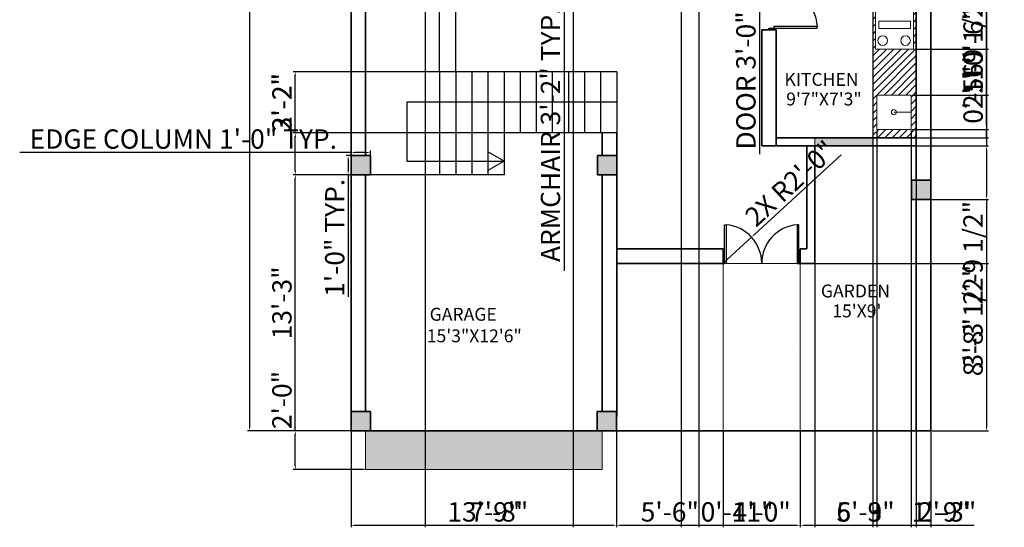
# Model space of a CAD drawing. Units: inches. Extents: x 2430 to 3058, y 1630 to 2396.
# Tile 1 of 4: x 2430 to 3042, y 1630 to 1945. Entities that reach past the tile are written whole.
import ezdxf

# ---------------------------------------------------------------- set-up
doc = ezdxf.new("R2010")
doc.units = ezdxf.units.IN
for name, color, linetype, lineweight in [('A-ANNO-DIMS', 7, 'Continuous', 18), ('A-AREA-IDEN', 131, 'Continuous', 18), ('A-COLS', 7, 'Continuous', 35), ('A-COLS-PATT', 1, 'Continuous', 13), ('A-DOOR', 40, 'Continuous', 25), ('A-FLOR-CASE', 7, 'Continuous', 25), ('A-FLOR-CASE-PATT', 131, 'Continuous', 13), ('A-FLOR-FIXT', 2, 'Continuous', 18), ('A-FLOR-STRS', 7, 'Continuous', 25), ('A-GLAZ', 131, 'Continuous', 18), ('A-GLAZ-PATT', 131, 'Continuous', 13), ('A-WALL', 7, 'Continuous', 35), ('L-PVMT', 7, 'Continuous', 18)]:
    doc.layers.add(name, color=color, linetype=linetype, lineweight=lineweight)
doc.layers.add('A-EQPM', color=33, linetype='Continuous', lineweight=18, true_color=0xb0a07d)
doc.layers.add('L-PVMT-PATT', color=241, linetype='Continuous', lineweight=13, true_color=0xf7abae)
doc.styles.get("Standard").update_dxf_attribs({"font": 'arial.ttf'})
doc.dimstyles.new('ISO-25', dxfattribs={"dimtxt": 12, "dimasz": 2.5, "dimexe": 1.25, "dimexo": 0.625, "dimtad": 1, "dimdec": 0, "dimlunit": 3, "dimtxsty": 'Standard', "dimcen": 2.5, "dimadec": 0, "dimazin": 0, "dimtfac": 1, "dimtdec": 0, "dimtmove": 0, "dimatfit": 3, "dimfxl": 1, "dimarcsym": 0})

# ---------------------------------------------------------------- blocks, each defined once
blk = doc.blocks.new('*D2')
at = {"layer": 'A-ANNO-DIMS', "color": 0, "lineweight": -2, "transparency": 16777216}
for p, q in [((2635.37, 2289.88), (2571.77, 2289.88)), ((2573.02, 2287.38), (2573.02, 1692.38)), ((2635.37, 1689.88), (2571.77, 1689.88))]:
    blk.add_line(p, q, dxfattribs=at)
at = {"layer": 'A-ANNO-DIMS', "color": 0, "transparency": 16777216}
for points in [[(2572.61, 2287.38), (2573.44, 2287.38), (2573.02, 2289.88)], [(2572.61, 1692.38), (2573.44, 1692.38), (2573.02, 1689.88)]]:
    blk.add_solid(points, dxfattribs=at)
at = {"layer": 'Defpoints', "color": 0, "transparency": 16777216}
for p in [(2636, 2289.88), (2573.02, 1689.88), (2636, 1689.88)]:
    blk.add_point(p, dxfattribs=at)
at = {"layer": 'A-ANNO-DIMS', "color": 0, "transparency": 16777216, "insert": (2566.27, 1989.88), "char_height": 12, "attachment_point": 5, "rotation": 90}
blk.add_mtext("50'", dxfattribs=at)
blk = doc.blocks.new('DOOR-30')
for p, q in [((0, 30), (0, 29)), ((0, 29), (30, 29)), ((3, 28), (3, 30)), ((30, 28), (3, 28)), ((30, 29), (30, 28)), ((0, 0), (0, 1)), ((0, 1), (3, 1)), ((3, 1), (3, 0))]:
    blk.add_line(p, q)
blk.add_arc((0.14, 30.86), 30, 275.47639, 354.52361)
blk = doc.blocks.new('COL-12x12-EDGE')
for p, q in [((12, 12), (0, 12)), ((0, 12), (0, 0)), ((0, 0), (12, 0))]:
    blk.add_line(p, q)
blk = doc.blocks.new('*D11')
at = {"layer": 'A-ANNO-DIMS', "color": 0, "lineweight": -2, "transparency": 16777216}
for p, q in [((2636, 1862.68), (2430.26, 1862.68)), ((2636, 1861.5), (2636, 1863.93)), ((2645.5, 1862.68), (2638.5, 1862.68)), ((2648, 1861.5), (2648, 1863.93))]:
    blk.add_line(p, q, dxfattribs=at)
at = {"layer": 'A-ANNO-DIMS', "color": 0, "transparency": 16777216}
for points in [[(2638.5, 1863.09), (2638.5, 1862.26), (2636, 1862.68)], [(2645.5, 1863.09), (2645.5, 1862.26), (2648, 1862.68)]]:
    blk.add_solid(points, dxfattribs=at)
at = {"layer": 'Defpoints', "color": 0, "transparency": 16777216}
for p in [(2636, 1862.68), (2636, 1860.88), (2648, 1860.88)]:
    blk.add_point(p, dxfattribs=at)
at = {"layer": 'A-ANNO-DIMS', "color": 0, "transparency": 16777216, "insert": (2531.88, 1869.51), "char_height": 12, "attachment_point": 5}
blk.add_mtext('EDGE COLUMN 1\'-0" TYP.', dxfattribs=at)
blk = doc.blocks.new('*D12')
at = {"layer": 'A-ANNO-DIMS', "color": 0, "lineweight": -2, "transparency": 16777216}
for p, q in [((2635.37, 1860.88), (2632.95, 1860.88)), ((2634.2, 1858.38), (2634.2, 1851.38)), ((2635.37, 1848.88), (2632.95, 1848.88)), ((2634.2, 1848.88), (2634.2, 1773.11))]:
    blk.add_line(p, q, dxfattribs=at)
at = {"layer": 'A-ANNO-DIMS', "color": 0, "transparency": 16777216}
for points in [[(2633.78, 1858.38), (2634.61, 1858.38), (2634.2, 1860.88)], [(2633.78, 1851.38), (2634.61, 1851.38), (2634.2, 1848.88)]]:
    blk.add_solid(points, dxfattribs=at)
at = {"layer": 'Defpoints', "color": 0, "transparency": 16777216}
for p in [(2636, 1860.88), (2634.2, 1848.88), (2636, 1848.88)]:
    blk.add_point(p, dxfattribs=at)
at = {"layer": 'A-ANNO-DIMS', "color": 0, "transparency": 16777216, "insert": (2627.44, 1809.74), "char_height": 12, "attachment_point": 5, "rotation": 90}
blk.add_mtext('1\'-0" TYP.', dxfattribs=at)
blk = doc.blocks.new('*D19')
at = {"layer": 'A-ANNO-DIMS', "color": 0, "lineweight": -2, "transparency": 16777216}
for p, q in [((2894.37, 2028.88), (2888.35, 2028.88)), ((2889.6, 2026.38), (2889.6, 1995.38)), ((2894.37, 1992.88), (2888.35, 1992.88)), ((2889.6, 1992.88), (2889.6, 1861.63))]:
    blk.add_line(p, q, dxfattribs=at)
at = {"layer": 'A-ANNO-DIMS', "color": 0, "transparency": 16777216}
for points in [[(2889.18, 2026.38), (2890.01, 2026.38), (2889.6, 2028.88)], [(2889.18, 1995.38), (2890.01, 1995.38), (2889.6, 1992.88)]]:
    blk.add_solid(points, dxfattribs=at)
at = {"layer": 'Defpoints', "color": 0, "transparency": 16777216}
for p in [(2895, 2028.88), (2889.6, 1992.88), (2895, 1992.88)]:
    blk.add_point(p, dxfattribs=at)
at = {"layer": 'A-ANNO-DIMS', "color": 0, "transparency": 16777216, "insert": (2882.76, 1926), "char_height": 12, "attachment_point": 5, "rotation": 90}
blk.add_mtext('DOOR 3\'-0" TYP.', dxfattribs=at)
blk = doc.blocks.new('*D25')
at = {"layer": 'A-ANNO-DIMS', "color": 0, "lineweight": -2, "transparency": 16777216}
for p, q in [((2773.33, 1998.82), (2767, 1998.82)), ((2768.25, 1996.32), (2768.25, 1963.32)), ((2773.33, 1960.82), (2767, 1960.82)), ((2768.25, 1960.82), (2768.25, 1789.16))]:
    blk.add_line(p, q, dxfattribs=at)
at = {"layer": 'A-ANNO-DIMS', "color": 0, "transparency": 16777216}
for points in [[(2767.83, 1996.32), (2768.67, 1996.32), (2768.25, 1998.82)], [(2767.83, 1963.32), (2768.67, 1963.32), (2768.25, 1960.82)]]:
    blk.add_solid(points, dxfattribs=at)
at = {"layer": 'Defpoints', "color": 0, "transparency": 16777216}
for p in [(2773.95, 1998.82), (2768.25, 1960.82), (2773.95, 1960.82)]:
    blk.add_point(p, dxfattribs=at)
at = {"layer": 'A-ANNO-DIMS', "color": 0, "transparency": 16777216, "insert": (2761.42, 1873.74), "char_height": 12, "attachment_point": 5, "rotation": 90}
blk.add_mtext('ARMCHAIR 3\'-2" TYP.', dxfattribs=at)
blk = doc.blocks.new('*D32')
at = {"layer": 'A-ANNO-DIMS', "color": 0, "lineweight": -2, "transparency": 16777216}
for p, q in [((2996.62, 1992.88), (3031.85, 1992.88)), ((3030.6, 1990.38), (3030.6, 1869.38)), ((2987.62, 1866.88), (3031.85, 1866.88))]:
    blk.add_line(p, q, dxfattribs=at)
at = {"layer": 'A-ANNO-DIMS', "color": 0, "transparency": 16777216}
for points in [[(3030.18, 1990.38), (3031.01, 1990.38), (3030.6, 1992.88)], [(3030.18, 1869.38), (3031.01, 1869.38), (3030.6, 1866.88)]]:
    blk.add_solid(points, dxfattribs=at)
at = {"layer": 'Defpoints', "color": 0, "transparency": 16777216}
for p in [(2996, 1992.88), (2987, 1866.88), (3030.6, 1866.88)]:
    blk.add_point(p, dxfattribs=at)
at = {"layer": 'A-ANNO-DIMS', "color": 0, "transparency": 16777216, "insert": (3023.84, 1929.88), "char_height": 12, "attachment_point": 5, "rotation": 90}
blk.add_mtext('10\'-6"', dxfattribs=at)
blk = doc.blocks.new('*D33')
at = {"layer": 'A-ANNO-DIMS', "color": 0, "lineweight": -2, "transparency": 16777216}
for p, q in [((2987.62, 1866.88), (3031.85, 1866.88)), ((3030.6, 1864.38), (3030.6, 1836.1)), ((2996.62, 1833.6), (3031.85, 1833.6)), ((3030.6, 1833.6), (3030.6, 1769.78))]:
    blk.add_line(p, q, dxfattribs=at)
at = {"layer": 'A-ANNO-DIMS', "color": 0, "transparency": 16777216}
for points in [[(3030.18, 1864.38), (3031.01, 1864.38), (3030.6, 1866.88)], [(3030.18, 1836.1), (3031.01, 1836.1), (3030.6, 1833.6)]]:
    blk.add_solid(points, dxfattribs=at)
at = {"layer": 'Defpoints', "color": 0, "transparency": 16777216}
for p in [(2987, 1866.88), (2996, 1833.6), (3030.6, 1833.6)]:
    blk.add_point(p, dxfattribs=at)
at = {"layer": 'A-ANNO-DIMS', "color": 0, "transparency": 16777216, "insert": (3023.77, 1800.44), "char_height": 12, "attachment_point": 5, "rotation": 90}
blk.add_mtext('2\'-9 1/2"', dxfattribs=at)
blk = doc.blocks.new('*D34')
at = {"layer": 'A-ANNO-DIMS', "color": 0, "lineweight": -2, "transparency": 16777216}
for p, q in [((2996.62, 1833.6), (3031.85, 1833.6)), ((3030.6, 1831.1), (3030.6, 1796.38)), ((2924.62, 1793.88), (3031.85, 1793.88)), ((3030.6, 1793.88), (3030.6, 1730.28))]:
    blk.add_line(p, q, dxfattribs=at)
at = {"layer": 'A-ANNO-DIMS', "color": 0, "transparency": 16777216}
for points in [[(3030.18, 1831.1), (3031.01, 1831.1), (3030.6, 1833.6)], [(3030.18, 1796.38), (3031.01, 1796.38), (3030.6, 1793.88)]]:
    blk.add_solid(points, dxfattribs=at)
at = {"layer": 'Defpoints', "color": 0, "transparency": 16777216}
for p in [(2996, 1833.6), (2924, 1793.88), (3030.6, 1793.88)]:
    blk.add_point(p, dxfattribs=at)
at = {"layer": 'A-ANNO-DIMS', "color": 0, "transparency": 16777216, "insert": (3023.76, 1760.83), "char_height": 12, "attachment_point": 5, "rotation": 90}
blk.add_mtext('3\'-3 1/2"', dxfattribs=at)
blk = doc.blocks.new('*D35')
at = {"layer": 'A-ANNO-DIMS', "color": 0, "lineweight": -2, "transparency": 16777216}
for p, q in [((2924.62, 1793.88), (3031.85, 1793.88)), ((3030.6, 1791.38), (3030.6, 1692.38)), ((2996.62, 1689.88), (3031.85, 1689.88))]:
    blk.add_line(p, q, dxfattribs=at)
at = {"layer": 'A-ANNO-DIMS', "color": 0, "transparency": 16777216}
for points in [[(3030.18, 1791.38), (3031.01, 1791.38), (3030.6, 1793.88)], [(3030.18, 1692.38), (3031.01, 1692.38), (3030.6, 1689.88)]]:
    blk.add_solid(points, dxfattribs=at)
at = {"layer": 'Defpoints', "color": 0, "transparency": 16777216}
for p in [(2924, 1793.88), (2996, 1689.88), (3030.6, 1689.88)]:
    blk.add_point(p, dxfattribs=at)
at = {"layer": 'A-ANNO-DIMS', "color": 0, "transparency": 16777216, "insert": (3023.84, 1741.88), "char_height": 12, "attachment_point": 5, "rotation": 90}
blk.add_mtext('8\'-8"', dxfattribs=at)
blk = doc.blocks.new('*D36')
at = {"layer": 'A-ANNO-DIMS', "color": 0, "lineweight": -2, "transparency": 16777216}
for p, q in [((2635.37, 1848.88), (2600.15, 1848.88)), ((2601.4, 1692.38), (2601.4, 1846.38)), ((2635.37, 1689.88), (2600.15, 1689.88))]:
    blk.add_line(p, q, dxfattribs=at)
at = {"layer": 'A-ANNO-DIMS', "color": 0, "transparency": 16777216}
for points in [[(2600.98, 1846.38), (2601.81, 1846.38), (2601.4, 1848.88)], [(2600.98, 1692.38), (2601.81, 1692.38), (2601.4, 1689.88)]]:
    blk.add_solid(points, dxfattribs=at)
at = {"layer": 'Defpoints', "color": 0, "transparency": 16777216}
for p in [(2601.4, 1848.88), (2636, 1848.88), (2636, 1689.88)]:
    blk.add_point(p, dxfattribs=at)
at = {"layer": 'A-ANNO-DIMS', "color": 0, "transparency": 16777216, "insert": (2594.64, 1769.38), "char_height": 12, "attachment_point": 5, "rotation": 90}
blk.add_mtext('13\'-3"', dxfattribs=at)
blk = doc.blocks.new('*D37')
at = {"layer": 'A-ANNO-DIMS', "color": 0, "lineweight": -2, "transparency": 16777216}
for p, q in [((2601.4, 1689.88), (2601.4, 1725.73)), ((2644.37, 1689.88), (2600.15, 1689.88)), ((2601.4, 1668.38), (2601.4, 1687.38)), ((2644.37, 1665.88), (2600.15, 1665.88))]:
    blk.add_line(p, q, dxfattribs=at)
at = {"layer": 'A-ANNO-DIMS', "color": 0, "transparency": 16777216}
for points in [[(2600.98, 1687.38), (2601.81, 1687.38), (2601.4, 1689.88)], [(2600.98, 1668.38), (2601.81, 1668.38), (2601.4, 1665.88)]]:
    blk.add_solid(points, dxfattribs=at)
at = {"layer": 'Defpoints', "color": 0, "transparency": 16777216}
for p in [(2601.4, 1689.88), (2645, 1689.88), (2645, 1665.88)]:
    blk.add_point(p, dxfattribs=at)
at = {"layer": 'A-ANNO-DIMS', "color": 0, "transparency": 16777216, "insert": (2594.64, 1709.05), "char_height": 12, "attachment_point": 5, "rotation": 90}
blk.add_mtext('2\'-0"', dxfattribs=at)
blk = doc.blocks.new('*D38')
at = {"layer": 'A-ANNO-DIMS', "color": 0, "lineweight": -2, "transparency": 16777216}
for p, q in [((2636, 1689.25), (2636, 1630.03)), ((2800.92, 1689.25), (2800.92, 1630.03)), ((2638.5, 1631.28), (2798.42, 1631.28))]:
    blk.add_line(p, q, dxfattribs=at)
at = {"layer": 'A-ANNO-DIMS', "color": 0, "transparency": 16777216}
for points in [[(2638.5, 1631.69), (2638.5, 1630.86), (2636, 1631.28)], [(2798.42, 1631.69), (2798.42, 1630.86), (2800.92, 1631.28)]]:
    blk.add_solid(points, dxfattribs=at)
at = {"layer": 'Defpoints', "color": 0, "transparency": 16777216}
for p in [(2636, 1689.88), (2800.92, 1689.88), (2800.92, 1631.28)]:
    blk.add_point(p, dxfattribs=at)
at = {"layer": 'A-ANNO-DIMS', "color": 0, "transparency": 16777216, "insert": (2718.46, 1638.03), "char_height": 12, "attachment_point": 5}
blk.add_mtext('13\'-9"', dxfattribs=at)
blk = doc.blocks.new('*D39')
at = {"layer": 'A-ANNO-DIMS', "color": 0, "lineweight": -2, "transparency": 16777216}
for p, q in [((2800.92, 1689.25), (2800.92, 1630.03)), ((2867, 1689.25), (2867, 1630.03)), ((2803.42, 1631.28), (2864.5, 1631.28))]:
    blk.add_line(p, q, dxfattribs=at)
at = {"layer": 'A-ANNO-DIMS', "color": 0, "transparency": 16777216}
for points in [[(2803.42, 1631.69), (2803.42, 1630.86), (2800.92, 1631.28)], [(2864.5, 1631.69), (2864.5, 1630.86), (2867, 1631.28)]]:
    blk.add_solid(points, dxfattribs=at)
at = {"layer": 'Defpoints', "color": 0, "transparency": 16777216}
for p in [(2800.92, 1689.88), (2867, 1689.88), (2867, 1631.28)]:
    blk.add_point(p, dxfattribs=at)
at = {"layer": 'A-ANNO-DIMS', "color": 0, "transparency": 16777216, "insert": (2833.96, 1638.03), "char_height": 12, "attachment_point": 5}
blk.add_mtext('5\'-6"', dxfattribs=at)
blk = doc.blocks.new('*D40')
at = {"layer": 'A-ANNO-DIMS', "color": 0, "lineweight": -2, "transparency": 16777216}
for p, q in [((2867, 1689.25), (2867, 1630.03)), ((2915, 1689.25), (2915, 1630.03)), ((2869.5, 1631.28), (2912.5, 1631.28))]:
    blk.add_line(p, q, dxfattribs=at)
at = {"layer": 'A-ANNO-DIMS', "color": 0, "transparency": 16777216}
for points in [[(2869.5, 1631.69), (2869.5, 1630.86), (2867, 1631.28)], [(2912.5, 1631.69), (2912.5, 1630.86), (2915, 1631.28)]]:
    blk.add_solid(points, dxfattribs=at)
at = {"layer": 'Defpoints', "color": 0, "transparency": 16777216}
for p in [(2867, 1689.88), (2915, 1689.88), (2915, 1631.28)]:
    blk.add_point(p, dxfattribs=at)
at = {"layer": 'A-ANNO-DIMS', "color": 0, "transparency": 16777216, "insert": (2891, 1638.03), "char_height": 12, "attachment_point": 5}
blk.add_mtext('4\'-0"', dxfattribs=at)
blk = doc.blocks.new('*D41')
at = {"layer": 'A-ANNO-DIMS', "color": 0, "lineweight": -2, "transparency": 16777216}
for p, q in [((2915, 1689.25), (2915, 1630.03)), ((2996, 1689.25), (2996, 1630.03)), ((2917.5, 1631.28), (2993.5, 1631.28))]:
    blk.add_line(p, q, dxfattribs=at)
at = {"layer": 'A-ANNO-DIMS', "color": 0, "transparency": 16777216}
for points in [[(2917.5, 1631.69), (2917.5, 1630.86), (2915, 1631.28)], [(2993.5, 1631.69), (2993.5, 1630.86), (2996, 1631.28)]]:
    blk.add_solid(points, dxfattribs=at)
at = {"layer": 'Defpoints', "color": 0, "transparency": 16777216}
for p in [(2915, 1689.88), (2996, 1689.88), (2996, 1631.28)]:
    blk.add_point(p, dxfattribs=at)
at = {"layer": 'A-ANNO-DIMS', "color": 0, "transparency": 16777216, "insert": (2955.5, 1638.03), "char_height": 12, "attachment_point": 5}
blk.add_mtext('6\'-9"', dxfattribs=at)
blk = doc.blocks.new('*D42')
at = {"layer": 'A-ANNO-DIMS', "color": 0, "lineweight": -2, "transparency": 16777216}
for p, q in [((2601.4, 1874.88), (2601.4, 1910.73)), ((2644.37, 1874.88), (2600.15, 1874.88)), ((2601.4, 1851.38), (2601.4, 1872.38)), ((2644.37, 1848.88), (2600.15, 1848.88))]:
    blk.add_line(p, q, dxfattribs=at)
at = {"layer": 'A-ANNO-DIMS', "color": 0, "transparency": 16777216}
for points in [[(2600.98, 1872.38), (2601.81, 1872.38), (2601.4, 1874.88)], [(2600.98, 1851.38), (2601.81, 1851.38), (2601.4, 1848.88)]]:
    blk.add_solid(points, dxfattribs=at)
at = {"layer": 'Defpoints', "color": 0, "transparency": 16777216}
for p in [(2601.4, 1874.88), (2645, 1874.88), (2645, 1848.88)]:
    blk.add_point(p, dxfattribs=at)
at = {"layer": 'A-ANNO-DIMS', "color": 0, "transparency": 16777216, "insert": (2594.75, 1894.05), "char_height": 12, "attachment_point": 5, "rotation": 90}
blk.add_mtext('2\'-2"', dxfattribs=at)
blk = doc.blocks.new('*D43')
at = {"layer": 'A-ANNO-DIMS', "color": 0, "lineweight": -2, "transparency": 16777216}
for p, q in [((2644.37, 1912.88), (2600.15, 1912.88)), ((2601.4, 1877.38), (2601.4, 1910.38)), ((2644.37, 1874.88), (2600.15, 1874.88))]:
    blk.add_line(p, q, dxfattribs=at)
at = {"layer": 'A-ANNO-DIMS', "color": 0, "transparency": 16777216}
for points in [[(2600.98, 1910.38), (2601.81, 1910.38), (2601.4, 1912.88)], [(2600.98, 1877.38), (2601.81, 1877.38), (2601.4, 1874.88)]]:
    blk.add_solid(points, dxfattribs=at)
at = {"layer": 'Defpoints', "color": 0, "transparency": 16777216}
for p in [(2601.4, 1912.88), (2645, 1912.88), (2645, 1874.88)]:
    blk.add_point(p, dxfattribs=at)
at = {"layer": 'A-ANNO-DIMS', "color": 0, "transparency": 16777216, "insert": (2594.64, 1893.88), "char_height": 12, "attachment_point": 5, "rotation": 90}
blk.add_mtext('3\'-2"', dxfattribs=at)
blk = doc.blocks.new('*D44')
at = {"layer": 'A-ANNO-DIMS', "color": 0, "lineweight": -2, "transparency": 16777216}
for p, q in [((2691, 1913.5), (2691, 2325.73)), ((2693.5, 2324.48), (2698.5, 2324.48)), ((2701, 1913.5), (2701, 2325.73)), ((2701, 2324.48), (2745.97, 2324.48))]:
    blk.add_line(p, q, dxfattribs=at)
at = {"layer": 'A-ANNO-DIMS', "color": 0, "transparency": 16777216}
for points in [[(2693.5, 2324.89), (2693.5, 2324.06), (2691, 2324.48)], [(2698.5, 2324.89), (2698.5, 2324.06), (2701, 2324.48)]]:
    blk.add_solid(points, dxfattribs=at)
at = {"layer": 'Defpoints', "color": 0, "transparency": 16777216}
for p in [(2701, 2324.48), (2691, 1912.88), (2701, 1912.88)]:
    blk.add_point(p, dxfattribs=at)
at = {"layer": 'A-ANNO-DIMS', "color": 0, "transparency": 16777216, "insert": (2724.73, 2331.23), "char_height": 12, "attachment_point": 5}
blk.add_mtext('0\'-10"', dxfattribs=at)
blk = doc.blocks.new('*D45')
at = {"layer": 'A-ANNO-DIMS', "color": 0, "lineweight": -2, "transparency": 16777216}
for p, q in [((2924, 1866.25), (2924, 1630.03)), ((2987, 1866.25), (2987, 1630.03)), ((2926.5, 1631.28), (2984.5, 1631.28))]:
    blk.add_line(p, q, dxfattribs=at)
at = {"layer": 'A-ANNO-DIMS', "color": 0, "transparency": 16777216}
for points in [[(2926.5, 1631.69), (2926.5, 1630.86), (2924, 1631.28)], [(2984.5, 1631.69), (2984.5, 1630.86), (2987, 1631.28)]]:
    blk.add_solid(points, dxfattribs=at)
at = {"layer": 'Defpoints', "color": 0, "transparency": 16777216}
for p in [(2924, 1866.88), (2987, 1866.88), (2987, 1631.28)]:
    blk.add_point(p, dxfattribs=at)
at = {"layer": 'A-ANNO-DIMS', "color": 0, "transparency": 16777216, "insert": (2955.5, 1638.03), "char_height": 12, "attachment_point": 5}
blk.add_mtext('5\'-3"', dxfattribs=at)
blk = doc.blocks.new('*D49')
at = {"layer": 'A-ANNO-DIMS', "color": 0, "lineweight": -2, "transparency": 16777216}
for p, q in [((2840.99, 2130.25), (2840.99, 1630.03)), ((2852, 2130.25), (2852, 1630.03)), ((2843.49, 1631.28), (2849.5, 1631.28)), ((2852, 1631.28), (2896.97, 1631.28))]:
    blk.add_line(p, q, dxfattribs=at)
at = {"layer": 'A-ANNO-DIMS', "color": 0, "transparency": 16777216}
for points in [[(2843.49, 1631.69), (2843.49, 1630.86), (2840.99, 1631.28)], [(2849.5, 1631.69), (2849.5, 1630.86), (2852, 1631.28)]]:
    blk.add_solid(points, dxfattribs=at)
at = {"layer": 'Defpoints', "color": 0, "transparency": 16777216}
for p in [(2840.99, 2130.88), (2852, 2130.88), (2852, 1631.28)]:
    blk.add_point(p, dxfattribs=at)
at = {"layer": 'A-ANNO-DIMS', "color": 0, "transparency": 16777216, "insert": (2875.73, 1638.03), "char_height": 12, "attachment_point": 5}
blk.add_mtext('0\'-11"', dxfattribs=at)
blk = doc.blocks.new('*D50')
at = {"layer": 'A-ANNO-DIMS', "color": 0, "lineweight": -2, "transparency": 16777216}
for p, q in [((2960, 1871.25), (2960, 1630.03)), ((2987, 1871.25), (2987, 1630.03)), ((2962.5, 1631.28), (2984.5, 1631.28)), ((2987, 1631.28), (3022.85, 1631.28))]:
    blk.add_line(p, q, dxfattribs=at)
at = {"layer": 'A-ANNO-DIMS', "color": 0, "transparency": 16777216}
for points in [[(2962.5, 1631.69), (2962.5, 1630.86), (2960, 1631.28)], [(2984.5, 1631.69), (2984.5, 1630.86), (2987, 1631.28)]]:
    blk.add_solid(points, dxfattribs=at)
at = {"layer": 'Defpoints', "color": 0, "transparency": 16777216}
for p in [(2960, 1871.88), (2987, 1871.88), (2987, 1631.28)]:
    blk.add_point(p, dxfattribs=at)
at = {"layer": 'A-ANNO-DIMS', "color": 0, "transparency": 16777216, "insert": (3006.17, 1638.03), "char_height": 12, "attachment_point": 5}
blk.add_mtext('2\'-3"', dxfattribs=at)
blk = doc.blocks.new('*D53')
at = {"layer": 'A-ANNO-DIMS', "color": 0, "lineweight": -2, "transparency": 16777216}
for p, q in [((2985.92, 1956.85), (3031.85, 1956.85)), ((3030.6, 1954.35), (3030.6, 1929.42)), ((2985.92, 1926.92), (3031.85, 1926.92)), ((3030.6, 1926.92), (3030.6, 1891.07))]:
    blk.add_line(p, q, dxfattribs=at)
at = {"layer": 'A-ANNO-DIMS', "color": 0, "transparency": 16777216}
for points in [[(3030.18, 1954.35), (3031.01, 1954.35), (3030.6, 1956.85)], [(3030.18, 1929.42), (3031.01, 1929.42), (3030.6, 1926.92)]]:
    blk.add_solid(points, dxfattribs=at)
at = {"layer": 'Defpoints', "color": 0, "transparency": 16777216}
for p in [(2985.3, 1956.85), (2985.3, 1926.92), (3030.6, 1926.92)]:
    blk.add_point(p, dxfattribs=at)
at = {"layer": 'A-ANNO-DIMS', "color": 0, "transparency": 16777216, "insert": (3023.84, 1907.75), "char_height": 12, "attachment_point": 5, "rotation": 90}
blk.add_mtext('2\'-6"', dxfattribs=at)
blk = doc.blocks.new('*D54')
at = {"layer": 'A-ANNO-DIMS', "color": 0, "lineweight": -2, "transparency": 16777216}
for p, q in [((2962.55, 1876.44), (2962.55, 1630.03)), ((2983.75, 1876.44), (2983.75, 1630.03)), ((2965.05, 1631.28), (2981.25, 1631.28)), ((2983.75, 1631.28), (3018.27, 1631.28))]:
    blk.add_line(p, q, dxfattribs=at)
at = {"layer": 'A-ANNO-DIMS', "color": 0, "transparency": 16777216}
for points in [[(2965.05, 1631.69), (2965.05, 1630.86), (2962.55, 1631.28)], [(2981.25, 1631.69), (2981.25, 1630.86), (2983.75, 1631.28)]]:
    blk.add_solid(points, dxfattribs=at)
at = {"layer": 'Defpoints', "color": 0, "transparency": 16777216}
for p in [(2962.55, 1877.06), (2983.75, 1877.06), (2983.75, 1631.28)]:
    blk.add_point(p, dxfattribs=at)
at = {"layer": 'A-ANNO-DIMS', "color": 0, "transparency": 16777216, "insert": (3002.26, 1638.03), "char_height": 12, "attachment_point": 5}
blk.add_mtext('1\'-9"', dxfattribs=at)
blk = doc.blocks.new('*D55')
at = {"layer": 'A-ANNO-DIMS', "color": 0, "lineweight": -2, "transparency": 16777216}
for p, q in [((3030.6, 1898.4), (3030.6, 1960.88)), ((2984.38, 1898.4), (3031.85, 1898.4)), ((3030.6, 1879.56), (3030.6, 1895.9)), ((2984.38, 1877.06), (3031.85, 1877.06))]:
    blk.add_line(p, q, dxfattribs=at)
at = {"layer": 'A-ANNO-DIMS', "color": 0, "transparency": 16777216}
for points in [[(3030.18, 1895.9), (3031.01, 1895.9), (3030.6, 1898.4)], [(3030.18, 1879.56), (3031.01, 1879.56), (3030.6, 1877.06)]]:
    blk.add_solid(points, dxfattribs=at)
at = {"layer": 'Defpoints', "color": 0, "transparency": 16777216}
for p in [(2983.75, 1898.4), (3030.6, 1898.4), (2983.75, 1877.06)]:
    blk.add_point(p, dxfattribs=at)
at = {"layer": 'A-ANNO-DIMS', "color": 0, "transparency": 16777216, "insert": (3023.77, 1930.89), "char_height": 12, "attachment_point": 5, "rotation": 90}
blk.add_mtext('1\'-9 1/2"', dxfattribs=at)
blk = doc.blocks.new('*D57')
at = {"layer": 'A-ANNO-DIMS', "color": 0, "lineweight": -2, "transparency": 16777216}
for p, q in [((3030.6, 1879.56), (3030.6, 1915.21)), ((2984.38, 1877.06), (3031.85, 1877.06)), ((3030.6, 1871.88), (3030.6, 1877.06)), ((2987.62, 1871.88), (3031.85, 1871.88)), ((3030.6, 1869.38), (3030.6, 1866.88))]:
    blk.add_line(p, q, dxfattribs=at)
at = {"layer": 'A-ANNO-DIMS', "color": 0, "transparency": 16777216}
for points in [[(3030.18, 1879.56), (3031.01, 1879.56), (3030.6, 1877.06)], [(3030.18, 1869.38), (3031.01, 1869.38), (3030.6, 1871.88)]]:
    blk.add_solid(points, dxfattribs=at)
at = {"layer": 'Defpoints', "color": 0, "transparency": 16777216}
for p in [(2983.75, 1877.06), (3030.6, 1877.06), (2987, 1871.88)]:
    blk.add_point(p, dxfattribs=at)
at = {"layer": 'A-ANNO-DIMS', "color": 0, "transparency": 16777216, "insert": (3023.84, 1898.64), "char_height": 12, "attachment_point": 5, "rotation": 90}
blk.add_mtext('0\'-5"', dxfattribs=at)
blk = doc.blocks.new('*D65')
at = {"layer": 'A-ANNO-DIMS', "color": 0, "lineweight": -2, "transparency": 16777216}
for p, q in [((2682, 1962.2), (2682, 1630.03)), ((2773.95, 1962.2), (2773.95, 1630.03)), ((2684.5, 1631.28), (2771.45, 1631.28))]:
    blk.add_line(p, q, dxfattribs=at)
at = {"layer": 'A-ANNO-DIMS', "color": 0, "transparency": 16777216}
for points in [[(2684.5, 1631.69), (2684.5, 1630.86), (2682, 1631.28)], [(2771.45, 1631.69), (2771.45, 1630.86), (2773.95, 1631.28)]]:
    blk.add_solid(points, dxfattribs=at)
at = {"layer": 'Defpoints', "color": 0, "transparency": 16777216}
for p in [(2682, 1962.82), (2773.95, 1962.82), (2773.95, 1631.28)]:
    blk.add_point(p, dxfattribs=at)
at = {"layer": 'A-ANNO-DIMS', "color": 0, "transparency": 16777216, "insert": (2727.97, 1638.03), "char_height": 12, "attachment_point": 5}
blk.add_mtext('7\'-8"', dxfattribs=at)
blk = doc.blocks.new('*D66')
at = {"layer": 'A-ANNO-DIMS', "color": 0, "lineweight": -2, "transparency": 16777216}
for p, q in [((2940.43, 1861.28), (2886.53, 1811.87)), ((2867, 1793.96), (2884.69, 1810.18))]:
    blk.add_line(p, q, dxfattribs=at)
at = {"layer": 'A-ANNO-DIMS', "color": 0, "transparency": 16777216}
blk.add_solid([(2886.25, 1812.18), (2886.81, 1811.56), (2884.69, 1810.18)], dxfattribs=at)
at = {"layer": 'Defpoints', "color": 0, "transparency": 16777216}
for p in [(2884.69, 1810.18), (2867, 1793.96)]:
    blk.add_point(p, dxfattribs=at)
at = {"layer": 'A-ANNO-DIMS', "color": 0, "transparency": 16777216, "insert": (2909.84, 1842.4), "char_height": 12, "attachment_point": 5, "rotation": 42.5117}
blk.add_mtext('2X R2\'-0"', dxfattribs=at)

msp = doc.modelspace()

# ---------------------------------------------------------------- hatches: boundary and pattern name
at = {"layer": 'A-COLS-PATT'}
h = msp.add_hatch(color=256, dxfattribs=at)
h.dxf.hatch_style = 1
h.paths.add_polyline_path([(2648, 1860.88), (2636, 1860.88), (2636, 1848.88), (2648, 1848.88)])
h = msp.add_hatch(color=256, dxfattribs=at)
h.dxf.hatch_style = 1
h.paths.add_polyline_path([(2801, 1860.88), (2789, 1860.88), (2789, 1848.88), (2801, 1848.88)])
h = msp.add_hatch(color=256, dxfattribs=at)
h.dxf.hatch_style = 1
h.paths.add_polyline_path([(2996, 1845.6), (2984, 1845.6), (2984, 1833.6), (2996, 1833.6)])
h = msp.add_hatch(color=256, dxfattribs=at)
h.dxf.hatch_style = 1
h.paths.add_polyline_path([(2648, 1701.88), (2636, 1701.88), (2636, 1689.88), (2648, 1689.88)])
h = msp.add_hatch(color=256, dxfattribs=at)
h.dxf.hatch_style = 1
h.paths.add_polyline_path([(2800.92, 1701.88), (2788.92, 1701.88), (2788.92, 1689.88), (2800.92, 1689.88)])
at = {"layer": 'A-FLOR-CASE-PATT'}
h = msp.add_hatch(dxfattribs=at)
h.set_pattern_fill('ANSI31', color=256)
h.paths.add_polyline_path([(2987, 1980.88), (2984, 1980.88), (2984, 1987.88), (2900, 1987.88), (2900, 1968.88), (2960, 1968.88), (2960, 1871.88), (2987, 1871.88)])
h.paths.add_polyline_path([(2961.68, 1956.85), (2985.3, 1956.85), (2985.3, 1926.92), (2961.68, 1926.92)], flags=16)
h.paths.add_polyline_path([(2969.08, 1951.68, -1), (2963.08, 1951.68, -1)], flags=0)
h.paths.add_polyline_path([(2963.83, 1944.18), (2983.44, 1944.18), (2983.44, 1939.79), (2963.83, 1939.79)], flags=0)
h.paths.add_polyline_path([(2983.32, 1951.68, -1), (2977.32, 1951.68, -1)], flags=0)
h.paths.add_polyline_path([(2969.08, 1932.19, -1), (2963.08, 1932.19, -1)], flags=0)
h.paths.add_polyline_path([(2983.32, 1932.19, -1), (2977.32, 1932.19, -1)], flags=0)
h.paths.add_polyline_path([(2962.55, 1898.4), (2983.75, 1898.4), (2983.75, 1877.06), (2962.55, 1877.06)], flags=16)
h.paths.add_polyline_path([(2974.72, 1887.73, -1), (2971.58, 1887.73, -1)], flags=0)
at = {"layer": 'A-GLAZ-PATT'}
h = msp.add_hatch(color=256, dxfattribs=at)
h.dxf.hatch_style = 1
h.paths.add_polyline_path([(2960, 1871.88), (2924, 1871.88), (2924, 1866.88), (2960, 1866.88)])
at = {"layer": 'L-PVMT-PATT'}
h = msp.add_hatch(dxfattribs=at)
h.set_pattern_fill('AR-CONC', color=256)
h.paths.add_polyline_path([(2915, 1793.88), (2914, 1793.88), (2913, 1793.88), (2867, 1793.88), (2867, 1698.88), (2915, 1698.88)])
h = msp.add_hatch(color=256, dxfattribs=at)
h.dxf.hatch_style = 1
h.paths.add_polyline_path([(2792, 1689.88), (2645, 1689.88), (2645, 1665.88), (2792, 1665.88)])

# ---------------------------------------------------------------- linework, layer by layer
at = {"layer": 'A-COLS'}
for p, q in [((2789, 1848.88), (2789, 1860.88)), ((2789, 1860.88), (2801, 1860.88)), ((2801, 1848.88), (2789, 1848.88)), ((2801, 1848.88), (2789, 1848.88))]:
    msp.add_line(p, q, dxfattribs=at)
at = {"layer": 'A-DOOR'}
for p, q in [((2868, 1793.88), (2868, 1817.88)), ((2868, 1817.88), (2869, 1817.88)), ((2869, 1817.88), (2869, 1793.88)), ((2914, 1817.88), (2913, 1817.88)), ((2913, 1817.88), (2913, 1793.88)), ((2914, 1793.88), (2914, 1817.88)), ((2867, 1793.88), (2868, 1793.88)), ((2869, 1793.88), (2867, 1793.88)), ((2913, 1793.88), (2914.5, 1793.88)), ((2915, 1793.88), (2914, 1793.88))]:
    msp.add_line(p, q, dxfattribs=at)
for centre, start, end in [((2867, 1793.96), 359.80074, 85.22016), ((2915, 1793.96), 94.77984, 180.19926)]:
    msp.add_arc(centre, 24, start, end, dxfattribs=at)
at = {"layer": 'A-EQPM'}
for points in [[(2961.68, 1956.85), (2985.3, 1956.85), (2985.3, 1926.92), (2961.68, 1926.92)], [(2963.83, 1944.18), (2983.44, 1944.18), (2983.44, 1939.79), (2963.83, 1939.79)]]:
    msp.add_lwpolyline(points, close=True, dxfattribs=at)
for centre in [(2966.08, 1932.19), (2980.32, 1932.19)]:
    msp.add_circle(centre, 3, dxfattribs=at)
at = {"layer": 'A-FLOR-CASE'}
msp.add_line((2960, 1968.88), (2960, 1871.88), dxfattribs=at)
at = {"layer": 'A-FLOR-FIXT'}
msp.add_line((2973.15, 1887.73), (2983.75, 1887.73), dxfattribs=at)
msp.add_lwpolyline([(2962.55, 1898.4), (2983.75, 1898.4), (2983.75, 1877.06), (2962.55, 1877.06)], close=True, dxfattribs=at)
msp.add_circle((2973.15, 1887.73), 1.57, dxfattribs=at)
at = {"layer": 'A-FLOR-STRS'}
for p, q in [((2801, 1912.88), (2645, 1912.88)), ((2691, 1912.88), (2691, 1848.88)), ((2701, 1912.88), (2701, 1848.88)), ((2711, 1912.88), (2711, 1848.88)), ((2721, 1912.88), (2721, 1848.88)), ((2731, 1912.88), (2731, 1848.88)), ((2741, 1912.88), (2741, 1874.88)), ((2751, 1912.88), (2751, 1874.88)), ((2761, 1912.88), (2761, 1874.88)), ((2771, 1912.88), (2771, 1874.88)), ((2781, 1912.88), (2781, 1874.88)), ((2791, 1912.88), (2791, 1874.88)), ((2801, 1912.88), (2801, 1874.88)), ((2801, 1893.88), (2670.61, 1893.88)), ((2670.61, 1893.88), (2670.61, 1857.36)), ((2801, 1874.88), (2645, 1874.88)), ((2731, 1857.36), (2721, 1863.14)), ((2670.61, 1857.36), (2731, 1857.36)), ((2731, 1857.36), (2721, 1851.59)), ((2731, 1848.88), (2645, 1848.88))]:
    msp.add_line(p, q, dxfattribs=at)
at = {"layer": 'A-GLAZ'}
for p, q in [((2924, 1871.88), (2924, 1866.88)), ((2960, 1871.88), (2960, 1866.88))]:
    msp.add_line(p, q, dxfattribs=at)
at = {"layer": 'A-WALL'}
for p, q in [((2645, 1860.88), (2645, 1989.88)), ((2987, 1980.88), (2987, 1845.6)), ((2891, 1938.88), (2900, 1938.88)), ((2891, 1938.88), (2891, 1866.88)), ((2900, 1938.88), (2900, 1866.88)), ((2792, 1860.88), (2792, 1874.88)), ((2801, 1698.88), (2801, 1874.88)), ((2900, 1871.88), (2987, 1871.88)), ((2891, 1866.88), (2987, 1866.88)), ((2919, 1866.88), (2919, 1802.88)), ((2924, 1866.88), (2924, 1793.88)), ((2645, 1701.88), (2645, 1848.88)), ((2792, 1701.88), (2792, 1848.88)), ((2987, 1833.6), (2987, 1689.88)), ((2867, 1802.88), (2801, 1802.88)), ((2867, 1802.88), (2867, 1793.88)), ((2915, 1802.88), (2915, 1793.88)), ((2919, 1802.88), (2915, 1802.88)), ((2867, 1793.88), (2801, 1793.88)), ((2924, 1793.88), (2915, 1793.88)), ((2801, 1698.88), (2800.92, 1698.88))]:
    msp.add_line(p, q, dxfattribs=at)
msp.add_lwpolyline([(2636, 2289.88), (2996, 2289.88), (2996, 1689.88), (2636, 1689.88)], close=True, dxfattribs=at)
at = {"layer": 'L-PVMT'}
for p, q in [((2867, 1793.88), (2867, 1689.88)), ((2867, 1793.88), (2915, 1793.88)), ((2915, 1793.88), (2915, 1689.88)), ((2645, 1689.88), (2645, 1665.88)), ((2792, 1665.88), (2792, 1689.88)), ((2645, 1665.88), (2792, 1665.88))]:
    msp.add_line(p, q, dxfattribs=at)

# ---------------------------------------------------------------- block references
at = {"layer": 'A-COLS'}
for p, rotation in [((2648, 1860.88), 180), ((2648, 1701.88), 180), ((2788.92, 1701.88), 270.0000000000029)]:
    msp.add_blockref('COL-12x12-EDGE', p, dxfattribs=dict(at, rotation=rotation))
msp.add_blockref('COL-12x12-EDGE', (2984, 1833.6), dxfattribs=at)
at = {"layer": 'A-DOOR', "extrusion": (0, 0, -1), "zscale": -1, "rotation": 180}
msp.add_blockref('DOOR-30', (-2895.5, 1968.88), dxfattribs=at)

# ---------------------------------------------------------------- texts
at = {"layer": 'A-AREA-IDEN'}
for tag, p in [('KITCHEN', (2905.13, 1904.08)), ('9\'7"X7\'3"', (2906.24, 1891.91)), ('GARDEN', (2927.78, 1772.74)), ("15'X9'", (2934.86, 1760.36)), ('GARAGE', (2684.84, 1758.27)), ('15\'3"X12\'6"', (2683.05, 1744.88))]:
    msp.add_attdef(tag, p, '', height=8, dxfattribs=at)

# ---------------------------------------------------------------- dimensions: what is measured, and where the dimension line sits
at = {"layer": 'A-ANNO-DIMS'}
for base, p1, p2, picture, middle in [((2701, 2324.48), (2691, 1912.88), (2701, 1912.88), '*D44', (2724.73, 2331.23)), ((2852, 1631.28), (2840.99, 2130.88), (2852, 2130.88), '*D49', (2875.73, 1638.03)), ((2773.9503, 1631.2777), (2681.9954, 1962.8232), (2773.9503, 1962.8232), '*D65', (2727.9729, 1638.0296)), ((2983.75, 1631.28), (2962.55, 1877.06), (2983.75, 1877.06), '*D54', (3002.26, 1638.03)), ((2987, 1631.28), (2960, 1871.88), (2987, 1871.88), '*D50', (3006.17, 1638.03)), ((2987, 1631.28), (2924, 1866.88), (2987, 1866.88), '*D45', (2955.5, 1638.03)), ((2800.92, 1631.28), (2636, 1689.88), (2800.92, 1689.88), '*D38', (2718.46, 1638.03)), ((2867, 1631.28), (2800.92, 1689.88), (2867, 1689.88), '*D39', (2833.96, 1638.03)), ((2915, 1631.28), (2867, 1689.88), (2915, 1689.88), '*D40', (2891, 1638.03)), ((2996, 1631.28), (2915, 1689.88), (2996, 1689.88), '*D41', (2955.5, 1638.03))]:
    dim = msp.add_linear_dim(base=base, p1=p1, p2=p2, dimstyle='ISO-25', override={"dimdec": 1, "dimlfac": 1, "dimrnd": 0, "dimzin": 1, "dimdsep": 46, "dimlunit": 4, "dimfrac": 2}, dxfattribs=at)
    dim.commit()
    dim.dimension.update_dxf_attribs({"geometry": picture, "text_midpoint": middle})
for base, p1, p2, override, picture, middle in [((2573.02, 1689.88), (2636, 2289.88), (2636, 1689.88), {"dimclrd": 0, "dimclre": 0, "dimclrt": 0}, '*D2', (2566.27, 1989.88)), ((3030.6, 1866.88), (2996, 1992.88), (2987, 1866.88), {"dimdec": 1, "dimlfac": 1, "dimrnd": 0, "dimzin": 1, "dimdsep": 46, "dimlunit": 4, "dimfrac": 2}, '*D32', (3023.84, 1929.88)), ((3030.6, 1898.4), (2983.75, 1877.06), (2983.75, 1898.4), {"dimdec": 1, "dimlfac": 1, "dimrnd": 0, "dimzin": 1, "dimdsep": 46, "dimlunit": 4, "dimfrac": 2}, '*D55', (3023.77, 1930.89)), ((3030.6, 1926.92), (2985.3, 1956.85), (2985.3, 1926.92), {"dimdec": 1, "dimlfac": 1, "dimrnd": 0, "dimzin": 1, "dimdsep": 46, "dimlunit": 4, "dimfrac": 2}, '*D53', (3023.84, 1907.75)), ((3030.6, 1877.06), (2987, 1871.88), (2983.75, 1877.06), {"dimdec": 1, "dimlfac": 1, "dimrnd": 0, "dimzin": 1, "dimdsep": 46, "dimlunit": 4, "dimfrac": 2}, '*D57', (3023.84, 1898.64)), ((2601.4, 1912.88), (2645, 1874.88), (2645, 1912.88), {"dimdec": 1, "dimlfac": 1, "dimrnd": 0, "dimzin": 1, "dimdsep": 46, "dimlunit": 4, "dimfrac": 2}, '*D43', (2594.64, 1893.88)), ((2601.4, 1874.88), (2645, 1848.88), (2645, 1874.88), {"dimdec": 1, "dimlfac": 1, "dimrnd": 0, "dimzin": 1, "dimdsep": 46, "dimlunit": 4, "dimfrac": 2}, '*D42', (2594.75, 1894.05)), ((3030.6, 1833.6), (2987, 1866.88), (2996, 1833.6), {"dimdec": 1, "dimlfac": 1, "dimrnd": 0, "dimzin": 1, "dimdsep": 46, "dimlunit": 4, "dimfrac": 2}, '*D33', (3023.77, 1800.44)), ((2601.4, 1848.88), (2636, 1689.88), (2636, 1848.88), {"dimdec": 1, "dimlfac": 1, "dimrnd": 0, "dimzin": 1, "dimdsep": 46, "dimlunit": 4, "dimfrac": 2}, '*D36', (2594.64, 1769.38)), ((3030.6, 1793.88), (2996, 1833.6), (2924, 1793.88), {"dimdec": 1, "dimlfac": 1, "dimrnd": 0, "dimzin": 1, "dimdsep": 46, "dimlunit": 4, "dimfrac": 2}, '*D34', (3023.76, 1760.83)), ((3030.6, 1689.88), (2924, 1793.88), (2996, 1689.88), {"dimdec": 1, "dimlfac": 1, "dimrnd": 0, "dimzin": 1, "dimdsep": 46, "dimlunit": 4, "dimfrac": 2}, '*D35', (3023.84, 1741.88)), ((2601.4, 1689.88), (2645, 1665.88), (2645, 1689.88), {"dimdec": 1, "dimlfac": 1, "dimrnd": 0, "dimzin": 1, "dimdsep": 46, "dimlunit": 4, "dimfrac": 2}, '*D37', (2594.64, 1709.05))]:
    dim = msp.add_linear_dim(base=base, p1=p1, p2=p2, angle=90, dimstyle='ISO-25', override=override, dxfattribs=at)
    dim.commit()
    dim.dimension.update_dxf_attribs({"geometry": picture, "text_midpoint": middle})
for base, p1, p2, angle, text, picture, middle in [((2889.6, 1992.88), (2895, 2028.88), (2895, 1992.88), 270, 'DOOR <> TYP.', '*D19', (2882.76, 1926)), ((2768.25, 1960.82), (2773.95, 1998.82), (2773.95, 1960.82), 270, 'ARMCHAIR <> TYP.', '*D25', (2761.42, 1873.74)), ((2636, 1862.68), (2648, 1860.88), (2636, 1860.88), 180, 'EDGE COLUMN <> TYP.', '*D11', (2531.88, 1869.51)), ((2634.2, 1848.88), (2636, 1860.88), (2636, 1848.88), 270, '<> TYP.', '*D12', (2627.44, 1809.74))]:
    dim = msp.add_linear_dim(base=base, p1=p1, p2=p2, angle=angle, text=text, dimstyle='ISO-25', override={"dimdec": 1, "dimlfac": 1, "dimrnd": 0, "dimzin": 1, "dimdsep": 46, "dimlunit": 4, "dimfrac": 2}, dxfattribs=at)
    dim.commit()
    dim.dimension.update_dxf_attribs({"geometry": picture, "text_midpoint": middle})
dim = msp.add_radius_dim(center=(2867, 1793.96), mpoint=(2884.69, 1810.18), text='2X <>', dimstyle='ISO-25', override={"dimdec": 1, "dimlfac": 1, "dimrnd": 0, "dimzin": 1, "dimdsep": 46, "dimlunit": 4, "dimfrac": 2}, dxfattribs=at)
dim.commit()
dim.dimension.update_dxf_attribs({"geometry": '*D66', "text_midpoint": (2909.84, 1842.4)})

doc.saveas('drawing.dxf')
